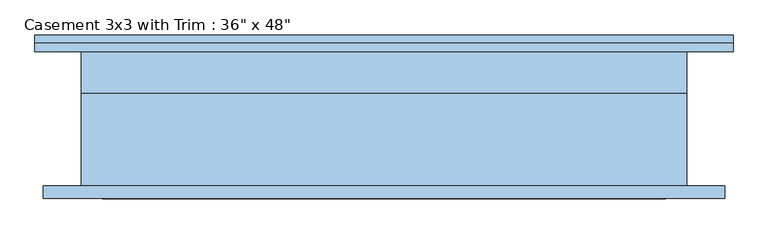
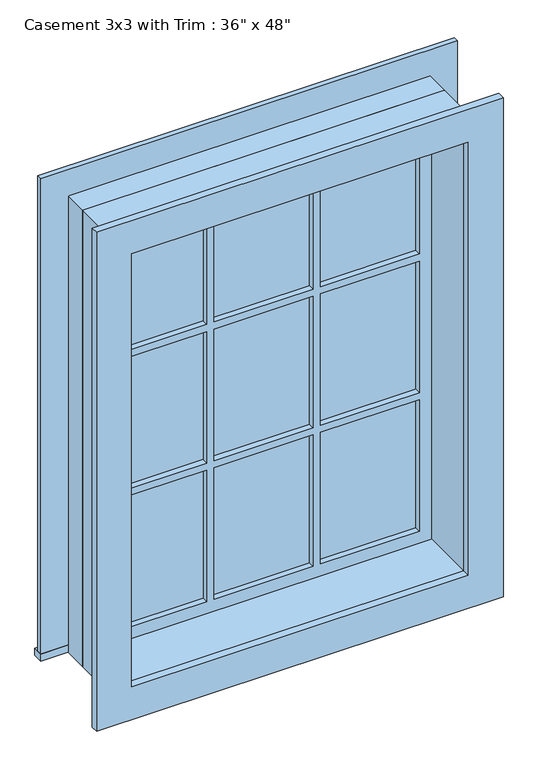
"""IFC4 building model written with IfcOpenShell, lengths in millimetres: window geometry."""

from ifc_helpers import new_model, si_unit, frame, origin, place, context, project, spatial, polyline, outline, extrude, source, transform, mapped, element, save


def window_29c06734(model_context):
    return source(origin(), model_context, "Body", "SweptSolid", [
        extrude(outline(polyline([(-527.05, 127.0), (527.05, 127.0), (527.05, 101.6), (-527.05, 101.6), (-527.05, 127.0)])), frame((0.0, 0.0, 914.4), z_axis=(0.0, 0.0, 1.0), x_axis=(1.0, 0.0, 0.0)), (0.0, 0.0, 1.0), 19.05),
        extrude(outline(polyline([(2114.55, -438.15), (2114.55, 438.15), (933.45, 438.15), (933.45, 527.05), (2203.45, 527.05), (2203.45, -527.05), (933.45, -527.05), (933.45, -438.15), (2114.55, -438.15)])), frame((0.0, 101.6, 0.0), z_axis=(0.0, 1.0, 0.0), x_axis=(0.0, 0.0, 1.0)), (0.0, 0.0, 1.0), 12.7),
        extrude(outline(polyline([(143.9333333, 66.675), (393.7, 66.675), (393.7, 53.975), (143.9333333, 53.975), (143.9333333, 66.675)])), frame((0.0, 0.0, 1718.7333333), z_axis=(0.0, 0.0, 1.0), x_axis=(1.0, 0.0, 0.0)), (0.0, 0.0, 1.0), 351.3666667),
        extrude(outline(polyline([(-124.8833333, 66.675), (124.8833333, 66.675), (124.8833333, 53.975), (-124.8833333, 53.975), (-124.8833333, 66.675)])), frame((0.0, 0.0, 1718.7333333), z_axis=(0.0, 0.0, 1.0), x_axis=(1.0, 0.0, 0.0)), (0.0, 0.0, 1.0), 351.3666667),
        extrude(outline(polyline([(-393.7, 66.675), (-143.9333333, 66.675), (-143.9333333, 53.975), (-393.7, 53.975), (-393.7, 66.675)])), frame((0.0, 0.0, 1718.7333333), z_axis=(0.0, 0.0, 1.0), x_axis=(1.0, 0.0, 0.0)), (0.0, 0.0, 1.0), 351.3666667),
        extrude(outline(polyline([(-393.7, 66.675), (-143.9333333, 66.675), (-143.9333333, 53.975), (-393.7, 53.975), (-393.7, 66.675)])), frame((0.0, 0.0, 1348.3166667), z_axis=(0.0, 0.0, 1.0), x_axis=(1.0, 0.0, 0.0)), (0.0, 0.0, 1.0), 351.3666667),
        extrude(outline(polyline([(-124.8833333, 66.675), (124.8833333, 66.675), (124.8833333, 53.975), (-124.8833333, 53.975), (-124.8833333, 66.675)])), frame((0.0, 0.0, 1348.3166667), z_axis=(0.0, 0.0, 1.0), x_axis=(1.0, 0.0, 0.0)), (0.0, 0.0, 1.0), 351.3666667),
        extrude(outline(polyline([(143.9333333, 66.675), (393.7, 66.675), (393.7, 53.975), (143.9333333, 53.975), (143.9333333, 66.675)])), frame((0.0, 0.0, 1348.3166667), z_axis=(0.0, 0.0, 1.0), x_axis=(1.0, 0.0, 0.0)), (0.0, 0.0, 1.0), 351.3666667),
        extrude(outline(polyline([(143.9333333, 66.675), (393.7, 66.675), (393.7, 53.975), (143.9333333, 53.975), (143.9333333, 66.675)])), frame((0.0, 0.0, 977.9), z_axis=(0.0, 0.0, 1.0), x_axis=(1.0, 0.0, 0.0)), (0.0, 0.0, 1.0), 351.3666667),
        extrude(outline(polyline([(-124.8833333, 66.675), (124.8833333, 66.675), (124.8833333, 53.975), (-124.8833333, 53.975), (-124.8833333, 66.675)])), frame((0.0, 0.0, 977.9), z_axis=(0.0, 0.0, 1.0), x_axis=(1.0, 0.0, 0.0)), (0.0, 0.0, 1.0), 351.3666667),
        extrude(outline(polyline([(-393.7, 66.675), (-143.9333333, 66.675), (-143.9333333, 53.975), (-393.7, 53.975), (-393.7, 66.675)])), frame((0.0, 0.0, 977.9), z_axis=(0.0, 0.0, 1.0), x_axis=(1.0, 0.0, 0.0)), (0.0, 0.0, 1.0), 351.3666667),
        extrude(outline(polyline([(2190.75, 514.35), (2190.75, -514.35), (857.25, -514.35), (857.25, 514.35), (2190.75, 514.35)]), holes=[polyline([(2101.85, 425.45), (946.15, 425.45), (946.15, -425.45), (2101.85, -425.45), (2101.85, 425.45)])]), frame((0.0, -120.65, 0.0), z_axis=(0.0, 1.0, 0.0), x_axis=(0.0, 0.0, 1.0)), (0.0, 0.0, 1.0), 19.05),
        extrude(outline(polyline([(2114.55, -438.15), (933.45, -438.15), (933.45, 438.15), (2114.55, 438.15), (2114.55, -438.15)]), holes=[polyline([(2070.1, -143.9333333), (1718.7333333, -143.9333333), (1718.7333333, -393.7), (2070.1, -393.7), (2070.1, -143.9333333)]), polyline([(1699.6833333, -143.9333333), (1348.3166667, -143.9333333), (1348.3166667, -393.7), (1699.6833333, -393.7), (1699.6833333, -143.9333333)]), polyline([(1329.2666667, -143.9333333), (977.9, -143.9333333), (977.9, -393.7), (1329.2666667, -393.7), (1329.2666667, -143.9333333)]), polyline([(2070.1, 124.8833333), (1718.7333333, 124.8833333), (1718.7333333, -124.8833333), (2070.1, -124.8833333), (2070.1, 124.8833333)]), polyline([(1699.6833333, 124.8833333), (1348.3166667, 124.8833333), (1348.3166667, -124.8833333), (1699.6833333, -124.8833333), (1699.6833333, 124.8833333)]), polyline([(1329.2666667, 124.8833333), (977.9, 124.8833333), (977.9, -124.8833333), (1329.2666667, -124.8833333), (1329.2666667, 124.8833333)]), polyline([(2070.1, 393.7), (1718.7333333, 393.7), (1718.7333333, 143.9333333), (2070.1, 143.9333333), (2070.1, 393.7)]), polyline([(1699.6833333, 393.7), (1348.3166667, 393.7), (1348.3166667, 143.9333333), (1699.6833333, 143.9333333), (1699.6833333, 393.7)]), polyline([(1329.2666667, 393.7), (977.9, 393.7), (977.9, 143.9333333), (1329.2666667, 143.9333333), (1329.2666667, 393.7)])]), frame((0.0, 38.1, 0.0), z_axis=(0.0, 1.0, 0.0), x_axis=(0.0, 0.0, 1.0)), (0.0, 0.0, 1.0), 44.45),
        extrude(outline(polyline([(2133.6, -457.2), (914.4, -457.2), (914.4, 457.2), (2133.6, 457.2), (2133.6, -457.2)]), holes=[polyline([(2101.85, -425.45), (2101.85, 425.45), (946.15, 425.45), (946.15, -425.45), (2101.85, -425.45)])]), frame((0.0, -101.6, 0.0), z_axis=(0.0, 1.0, 0.0), x_axis=(0.0, 0.0, 1.0)), (0.0, 0.0, 1.0), 139.7),
        extrude(outline(polyline([(2133.6, 457.2), (2133.6, -457.2), (914.4, -457.2), (914.4, 457.2), (2133.6, 457.2)]), holes=[polyline([(2114.55, 438.15), (933.45, 438.15), (933.45, -438.15), (2114.55, -438.15), (2114.55, 438.15)])]), frame((0.0, 38.1, 0.0), z_axis=(0.0, 1.0, 0.0), x_axis=(0.0, 0.0, 1.0)), (0.0, 0.0, 1.0), 63.5),
    ])


if __name__ == "__main__":
    model = new_model("IFC4")
    model_context = context("Model", 3, world=origin())
    ifc_project = project(units=[si_unit("LENGTHUNIT", "METRE", prefix="MILLI")], contexts=[model_context])
    site = spatial("IfcSite", under=ifc_project)
    building = spatial("IfcBuilding", under=site)
    placement = place(None, origin())
    window_shape = window_29c06734(model_context)
    element("IfcWindow", 1, ObjectType="Casement 3x3 with Trim : 36\" x 48\"", at=placement, inside=building, context=model_context, shape_type="MappedRepresentation", body=[
        mapped(window_shape, transform((0.0, 0.0, 0.0), x_axis=(1.0, 0.0, 0.0), y_axis=(0.0, 1.0, 0.0), z_axis=(0.0, 0.0, 1.0))),
    ])
    save(model, "model.ifc")

# Revit data of these elements
# Type "Casement 3x3 with Trim : 36\" x 48\""
#   Type Mark = "20"
#   Construction Type Id = "GSP4R"
#   Assembly Code = "B2020100"
#   Analytic Construction = "1/8 in Pilkington single glazing"
#   Visual Light Transmittance = 0.9
#   Solar Heat Gain Coefficient = 0.78
#   Heat Transfer Coefficient (U) = 0.6496 BTU/(h·ft²·°F)
#   Height = 4' - 0"
#   Default Sill Height = 3' - 0"
#   Trim Projection - Ext. = 0' - 0 1/2"
#   Trim Projection - Int. = 0' - 0 3/4"
#   Trim Width - Exterior = 0' - 3 1/2"
#   Trim Width - Interior = 0' - 3 1/2"
#   Width = 3' - 0"
#   Window Inset = 0' - 0 3/4"
#   Define Thermal Properties by = 1
#   Glass Pane Material = Glass
#   Sash Material = Sash
#   Trim Exterior Material = Trim
#   Trim Interior Material = Trim
#   Wall Closure = (empty or 0)
# Element 1 (IfcWindow, "Casement 3x3 with Trim : 36\" x 48\"")
#   Materials on its faces: "Sash", "Glass", "Trim"
# Materials
#   "Glass": class "Glass", colour RGB 0 128 192, transparency 0.75, Description = "Soda Lime Glass", Cost = 0
#   "Sash": class "Wood", colour RGB 224 178 126, transparency 0
#   "Trim": class "Wood", colour RGB 224 178 126, transparency 0
